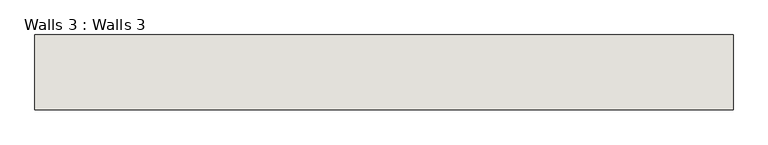
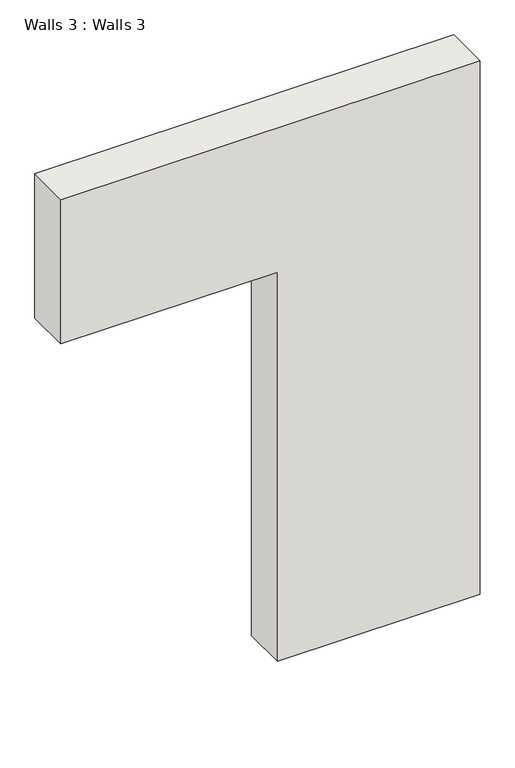
"""IFC4 building model written with IfcOpenShell, lengths in millimetres: wall geometry, Walls 3 : Walls 3."""

from ifc_helpers import new_model, si_unit, frame, origin, place, context, project, spatial, polyline, outline, extrude, source, transform, mapped, element, save


def walls_3_walls_3_8b246382(model_context):
    return source(origin(), model_context, "Body", "SweptSolid", [
        extrude(outline(polyline([(3830.5245478, -12950.1371903), (3830.5245478, -15798.6897324), (2794.0, -15798.6897324), (2794.0, -14325.4897324), (0.0, -14325.4897324), (0.0, -12950.1371903), (3830.5245478, -12950.1371903)])), frame((0.0, -3695.7180898, 0.0), z_axis=(0.0, 1.0, 0.0), x_axis=(0.0, 0.0, 1.0)), (0.0, 0.0, 1.0), 304.8),
    ])


if __name__ == "__main__":
    model = new_model("IFC4")
    model_context = context("Model", 3, world=origin())
    ifc_project = project(units=[si_unit("LENGTHUNIT", "METRE", prefix="MILLI")], contexts=[model_context])
    site = spatial("IfcSite", under=ifc_project)
    building = spatial("IfcBuilding", under=site)
    placement = place(None, origin())
    walls_3_walls_3_shape = walls_3_walls_3_8b246382(model_context)
    element("IfcWall", 1, ObjectType="Walls 3 : Walls 3", at=placement, inside=building, context=model_context, shape_type="MappedRepresentation", body=[
        mapped(walls_3_walls_3_shape, transform((0.0, 0.0, 0.0), x_axis=(1.0, 0.0, 0.0), y_axis=(0.0, 1.0, 0.0), z_axis=(0.0, 0.0, 1.0))),
    ])
    save(model, "model.ifc")

# Revit data of these elements
# Element 1 (IfcWall, "Walls 3 : Walls 3")
#   Materials on its faces: "Default Wall"
# Materials
#   "Default Wall": colour RGB 80 80 80, transparency 0
